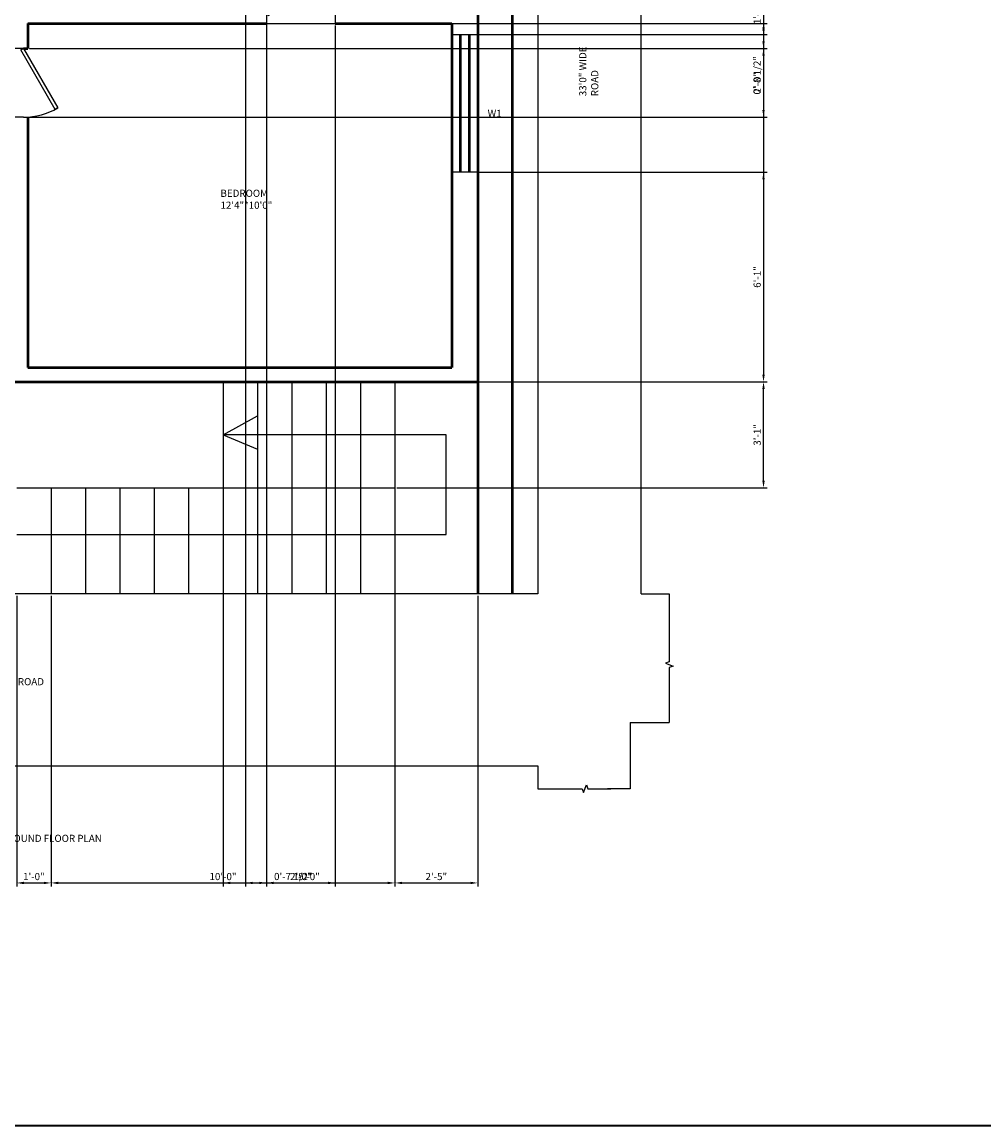
# Model space of a CAD drawing. Units: inches. Extents: x 2020 to 7901, y 1581 to 3943.
# Tile 3 of 17: x 2539 to 2875, y 1581 to 1966. Entities that reach past the tile are written whole.
import ezdxf

# ---------------------------------------------------------------- set-up
doc = ezdxf.new("R2010")
doc.units = ezdxf.units.IN
for name, color, linetype, lineweight in [('A-ANNO-DIMS', 2, 'Continuous', 18), ('A-ANNO-TEXT', 7, 'Continuous', 18), ('A-ANNO-TTLB', 7, 'Continuous', 35), ('A-AREA-IDEN', 3, 'Continuous', 18), ('A-DOOR', 4, 'Continuous', 25), ('A-FLOR-STRS', 3, 'Continuous', 25), ('A-GLAZ', 4, 'Continuous', 25), ('A-WALL', 7, 'Continuous', 50), ('C-PROP', 6, 'Continuous', 25)]:
    doc.layers.add(name, color=color, linetype=linetype, lineweight=lineweight)
doc.styles.get("Standard").update_dxf_attribs({"font": 'arial.ttf'})
doc.dimstyles.new('ISO-25', dxfattribs={"dimtxt": 2.5, "dimasz": 2.5, "dimexe": 1.25, "dimexo": 0.625, "dimtad": 1, "dimdec": 1, "dimlunit": 3, "dimtxsty": 'Standard', "dimcen": 2.5, "dimadec": 0, "dimazin": 0, "dimtfac": 1, "dimtdec": 1, "dimtmove": 0, "dimatfit": 3, "dimfxl": 1, "dimarcsym": 0})

# ---------------------------------------------------------------- blocks, each defined once
blk = doc.blocks.new('*U2')
for p, q in [((0, 0), (0, -6)), ((40, 0), (40, -6))]:
    blk.add_line(p, q)
blk.add_lwpolyline([(0, 0), (34.64, 20), (35.52, 18.48), (0.87, -1.52)], close=True)
blk.add_arc((0, 0), 40, 0, 30)
blk = doc.blocks.new('WIN-1200')
for p, q in [((0, 9), (48, 9)), ((0, 0), (0, 9)), ((48, 9), (48, 0)), ((48, 0), (0, 0))]:
    blk.add_line(p, q)
blk = doc.blocks.new('*D36')
at = {"layer": 'A-ANNO-DIMS', "color": 0, "lineweight": -2, "transparency": 16777216}
for p, q in [((2698.59, 1982.22), (2798.95, 1982.22)), ((2797.7, 1979.72), (2797.7, 1964)), ((2698.59, 1961.5), (2798.95, 1961.5))]:
    blk.add_line(p, q, dxfattribs=at)
at = {"layer": 'A-ANNO-DIMS', "color": 0, "transparency": 16777216}
for points in [[(2797.28, 1979.72), (2798.12, 1979.72), (2797.7, 1982.22)], [(2797.28, 1964), (2798.12, 1964), (2797.7, 1961.5)]]:
    blk.add_solid(points, dxfattribs=at)
at = {"layer": 'DEFPOINTS', "color": 0, "transparency": 16777216}
for p in [(2697.96, 1982.22), (2697.96, 1961.5), (2797.7, 1961.5)]:
    blk.add_point(p, dxfattribs=at)
at = {"layer": 'A-ANNO-DIMS', "color": 0, "transparency": 16777216, "insert": (2795.78, 1971.86), "char_height": 2.5, "attachment_point": 5, "rotation": 90}
blk.add_mtext('1\'-8 1/2"', dxfattribs=at)
blk = doc.blocks.new('*D37')
at = {"layer": 'A-ANNO-DIMS', "color": 0, "lineweight": -2, "transparency": 16777216}
for p, q in [((2698.59, 1913.5), (2798.95, 1913.5)), ((2797.7, 1911), (2797.7, 1842.84)), ((2698.59, 1840.34), (2798.95, 1840.34))]:
    blk.add_line(p, q, dxfattribs=at)
at = {"layer": 'A-ANNO-DIMS', "color": 0, "transparency": 16777216}
for points in [[(2797.28, 1911), (2798.12, 1911), (2797.7, 1913.5)], [(2797.28, 1842.84), (2798.12, 1842.84), (2797.7, 1840.34)]]:
    blk.add_solid(points, dxfattribs=at)
at = {"layer": 'DEFPOINTS', "color": 0, "transparency": 16777216}
for p in [(2697.96, 1913.5), (2697.96, 1840.34), (2797.7, 1840.34)]:
    blk.add_point(p, dxfattribs=at)
at = {"layer": 'A-ANNO-DIMS', "color": 0, "transparency": 16777216, "insert": (2795.8, 1876.92), "char_height": 2.5, "attachment_point": 5, "rotation": 90}
blk.add_mtext('6\'-1"', dxfattribs=at)
blk = doc.blocks.new('*D39')
at = {"layer": 'A-ANNO-DIMS', "color": 0, "lineweight": -2, "transparency": 16777216}
for p, q in [((2537.1, 1765.71), (2537.1, 1664.26)), ((2549.1, 1765.71), (2549.1, 1664.26)), ((2539.6, 1665.51), (2546.6, 1665.51))]:
    blk.add_line(p, q, dxfattribs=at)
at = {"layer": 'A-ANNO-DIMS', "color": 0, "transparency": 16777216}
for points in [[(2539.6, 1665.92), (2539.6, 1665.09), (2537.1, 1665.51)], [(2546.6, 1665.92), (2546.6, 1665.09), (2549.1, 1665.51)]]:
    blk.add_solid(points, dxfattribs=at)
at = {"layer": 'DEFPOINTS', "color": 0, "transparency": 16777216}
for p in [(2537.1, 1766.34), (2549.1, 1766.34), (2549.1, 1665.51)]:
    blk.add_point(p, dxfattribs=at)
at = {"layer": 'A-ANNO-DIMS', "color": 0, "transparency": 16777216, "insert": (2543.1, 1667.41), "char_height": 2.5, "attachment_point": 5}
blk.add_mtext('1\'-0"', dxfattribs=at)
blk = doc.blocks.new('*D40')
at = {"layer": 'A-ANNO-DIMS', "color": 0, "lineweight": -2, "transparency": 16777216}
for p, q in [((2549.1, 1765.71), (2549.1, 1664.26)), ((2669.1, 1765.71), (2669.1, 1664.26)), ((2551.6, 1665.51), (2666.6, 1665.51))]:
    blk.add_line(p, q, dxfattribs=at)
at = {"layer": 'A-ANNO-DIMS', "color": 0, "transparency": 16777216}
for points in [[(2551.6, 1665.92), (2551.6, 1665.09), (2549.1, 1665.51)], [(2666.6, 1665.92), (2666.6, 1665.09), (2669.1, 1665.51)]]:
    blk.add_solid(points, dxfattribs=at)
at = {"layer": 'DEFPOINTS', "color": 0, "transparency": 16777216}
for p in [(2549.1, 1766.34), (2669.1, 1766.34), (2669.1, 1665.51)]:
    blk.add_point(p, dxfattribs=at)
at = {"layer": 'A-ANNO-DIMS', "color": 0, "transparency": 16777216, "insert": (2609.1, 1667.41), "char_height": 2.5, "attachment_point": 5}
blk.add_mtext('10\'-0"', dxfattribs=at)
blk = doc.blocks.new('*D96')
at = {"layer": 'A-ANNO-DIMS', "color": 0, "lineweight": -2, "transparency": 16777216}
for p, q in [((2698.59, 2214.34), (2798.95, 2214.34)), ((2797.7, 2211.84), (2797.7, 1842.84)), ((2698.59, 1840.34), (2798.95, 1840.34))]:
    blk.add_line(p, q, dxfattribs=at)
at = {"layer": 'A-ANNO-DIMS', "color": 0, "transparency": 16777216}
for points in [[(2797.28, 2211.84), (2798.12, 2211.84), (2797.7, 2214.34)], [(2797.28, 1842.84), (2798.12, 1842.84), (2797.7, 1840.34)]]:
    blk.add_solid(points, dxfattribs=at)
at = {"layer": 'DEFPOINTS', "color": 0, "transparency": 16777216}
for p in [(2697.96, 2214.34), (2697.96, 1840.34), (2797.7, 1840.34)]:
    blk.add_point(p, dxfattribs=at)
at = {"layer": 'A-ANNO-DIMS', "color": 0, "transparency": 16777216, "insert": (2795.8, 2027.34), "char_height": 2.5, "attachment_point": 5, "rotation": 90}
blk.add_mtext('31\'-2"', dxfattribs=at)
blk = doc.blocks.new('*D112')
at = {"layer": 'A-ANNO-DIMS', "color": 0, "lineweight": -2, "transparency": 16777216}
for p, q in [((2541.59, 1965.34), (2798.95, 1965.34)), ((2797.7, 1962.84), (2797.7, 1959.17)), ((2541.59, 1956.67), (2798.95, 1956.67)), ((2797.7, 1956.67), (2797.7, 1940.45))]:
    blk.add_line(p, q, dxfattribs=at)
at = {"layer": 'A-ANNO-DIMS', "color": 0, "transparency": 16777216}
for points in [[(2797.28, 1962.84), (2798.12, 1962.84), (2797.7, 1965.34)], [(2797.28, 1959.17), (2798.12, 1959.17), (2797.7, 1956.67)]]:
    blk.add_solid(points, dxfattribs=at)
at = {"layer": 'DEFPOINTS', "color": 0, "transparency": 16777216}
for p in [(2540.96, 1965.34), (2540.96, 1956.67), (2797.7, 1956.67)]:
    blk.add_point(p, dxfattribs=at)
at = {"layer": 'A-ANNO-DIMS', "color": 0, "transparency": 16777216, "insert": (2795.78, 1947.31), "char_height": 2.5, "attachment_point": 5, "rotation": 90}
blk.add_mtext('0\'-8 1/2"', dxfattribs=at)
blk = doc.blocks.new('*D113')
at = {"layer": 'A-ANNO-DIMS', "color": 0, "lineweight": -2, "transparency": 16777216}
for p, q in [((2541.59, 1956.67), (2798.95, 1956.67)), ((2797.7, 1954.17), (2797.7, 1935.21)), ((2541.59, 1932.71), (2798.95, 1932.71))]:
    blk.add_line(p, q, dxfattribs=at)
at = {"layer": 'A-ANNO-DIMS', "color": 0, "transparency": 16777216}
for points in [[(2797.28, 1954.17), (2798.12, 1954.17), (2797.7, 1956.67)], [(2797.28, 1935.21), (2798.12, 1935.21), (2797.7, 1932.71)]]:
    blk.add_solid(points, dxfattribs=at)
at = {"layer": 'DEFPOINTS', "color": 0, "transparency": 16777216}
for p in [(2540.96, 1956.67), (2540.96, 1932.71), (2797.7, 1932.71)]:
    blk.add_point(p, dxfattribs=at)
at = {"layer": 'A-ANNO-DIMS', "color": 0, "transparency": 16777216, "insert": (2795.8, 1944.69), "char_height": 2.5, "attachment_point": 5, "rotation": 90}
blk.add_mtext('2\'-0"', dxfattribs=at)
blk = doc.blocks.new('*D116')
at = {"layer": 'A-ANNO-DIMS', "color": 0, "lineweight": -2, "transparency": 16777216}
for p, q in [((2616.96, 1969.71), (2616.96, 1664.26)), ((2624.26, 1969.71), (2624.26, 1664.26)), ((2619.46, 1665.51), (2621.76, 1665.51)), ((2624.26, 1665.51), (2640.48, 1665.51))]:
    blk.add_line(p, q, dxfattribs=at)
at = {"layer": 'A-ANNO-DIMS', "color": 0, "transparency": 16777216}
for points in [[(2619.46, 1665.92), (2619.46, 1665.09), (2616.96, 1665.51)], [(2621.76, 1665.92), (2621.76, 1665.09), (2624.26, 1665.51)]]:
    blk.add_solid(points, dxfattribs=at)
at = {"layer": 'DEFPOINTS', "color": 0, "transparency": 16777216}
for p in [(2616.96, 1970.34), (2624.26, 1970.34), (2624.26, 1665.51)]:
    blk.add_point(p, dxfattribs=at)
at = {"layer": 'A-ANNO-DIMS', "color": 0, "transparency": 16777216, "insert": (2633.62, 1667.43), "char_height": 2.5, "attachment_point": 5}
blk.add_mtext('0\'-7 1/2"', dxfattribs=at)
blk = doc.blocks.new('*D117')
at = {"layer": 'A-ANNO-DIMS', "color": 0, "lineweight": -2, "transparency": 16777216}
for p, q in [((2624.26, 1964.71), (2624.26, 1664.26)), ((2648.26, 1964.71), (2648.26, 1664.26)), ((2626.76, 1665.51), (2645.76, 1665.51))]:
    blk.add_line(p, q, dxfattribs=at)
at = {"layer": 'A-ANNO-DIMS', "color": 0, "transparency": 16777216}
for points in [[(2626.76, 1665.92), (2626.76, 1665.09), (2624.26, 1665.51)], [(2645.76, 1665.92), (2645.76, 1665.09), (2648.26, 1665.51)]]:
    blk.add_solid(points, dxfattribs=at)
at = {"layer": 'DEFPOINTS', "color": 0, "transparency": 16777216}
for p in [(2624.26, 1965.34), (2648.26, 1965.34), (2648.26, 1665.51)]:
    blk.add_point(p, dxfattribs=at)
at = {"layer": 'A-ANNO-DIMS', "color": 0, "transparency": 16777216, "insert": (2636.26, 1667.41), "char_height": 2.5, "attachment_point": 5}
blk.add_mtext('2\'-0"', dxfattribs=at)
blk = doc.blocks.new('*D119')
at = {"layer": 'A-ANNO-DIMS', "color": 0, "lineweight": -2, "transparency": 16777216}
for p, q in [((2609.1, 1839.71), (2609.1, 1664.26)), ((2669.1, 1839.71), (2669.1, 1664.26)), ((2611.6, 1665.51), (2666.6, 1665.51))]:
    blk.add_line(p, q, dxfattribs=at)
at = {"layer": 'A-ANNO-DIMS', "color": 0, "transparency": 16777216}
for points in [[(2611.6, 1665.92), (2611.6, 1665.09), (2609.1, 1665.51)], [(2666.6, 1665.92), (2666.6, 1665.09), (2669.1, 1665.51)]]:
    blk.add_solid(points, dxfattribs=at)
at = {"layer": 'DEFPOINTS', "color": 0, "transparency": 16777216}
for p in [(2609.1, 1840.34), (2669.1, 1840.34), (2669.1, 1665.51)]:
    blk.add_point(p, dxfattribs=at)
at = {"layer": 'A-ANNO-DIMS', "color": 0, "transparency": 16777216, "insert": (2639.1, 1667.41), "char_height": 2.5, "attachment_point": 5}
blk.add_mtext('5\'-0"', dxfattribs=at)
blk = doc.blocks.new('*D120')
at = {"layer": 'A-ANNO-DIMS', "color": 0, "lineweight": -2, "transparency": 16777216}
for p, q in [((2669.73, 1840.34), (2798.95, 1840.34)), ((2797.7, 1805.84), (2797.7, 1837.84)), ((2669.73, 1803.34), (2798.95, 1803.34))]:
    blk.add_line(p, q, dxfattribs=at)
at = {"layer": 'A-ANNO-DIMS', "color": 0, "transparency": 16777216}
for points in [[(2797.28, 1837.84), (2798.12, 1837.84), (2797.7, 1840.34)], [(2797.28, 1805.84), (2798.12, 1805.84), (2797.7, 1803.34)]]:
    blk.add_solid(points, dxfattribs=at)
at = {"layer": 'DEFPOINTS', "color": 0, "transparency": 16777216}
for p in [(2669.1, 1840.34), (2797.7, 1840.34), (2669.1, 1803.34)]:
    blk.add_point(p, dxfattribs=at)
at = {"layer": 'A-ANNO-DIMS', "color": 0, "transparency": 16777216, "insert": (2795.8, 1821.84), "char_height": 2.5, "attachment_point": 5, "rotation": 90}
blk.add_mtext('3\'-1"', dxfattribs=at)
blk = doc.blocks.new('*D121')
at = {"layer": 'A-ANNO-DIMS', "color": 0, "lineweight": -2, "transparency": 16777216}
for p, q in [((2669.1, 1765.71), (2669.1, 1664.26)), ((2697.96, 1765.71), (2697.96, 1664.26)), ((2671.6, 1665.51), (2695.46, 1665.51))]:
    blk.add_line(p, q, dxfattribs=at)
at = {"layer": 'A-ANNO-DIMS', "color": 0, "transparency": 16777216}
for points in [[(2671.6, 1665.92), (2671.6, 1665.09), (2669.1, 1665.51)], [(2695.46, 1665.92), (2695.46, 1665.09), (2697.96, 1665.51)]]:
    blk.add_solid(points, dxfattribs=at)
at = {"layer": 'DEFPOINTS', "color": 0, "transparency": 16777216}
for p in [(2669.1, 1766.34), (2697.96, 1766.34), (2697.96, 1665.51)]:
    blk.add_point(p, dxfattribs=at)
at = {"layer": 'A-ANNO-DIMS', "color": 0, "transparency": 16777216, "insert": (2683.53, 1667.41), "char_height": 2.5, "attachment_point": 5}
blk.add_mtext('2\'-5"', dxfattribs=at)

msp = doc.modelspace()

# ---------------------------------------------------------------- linework, layer by layer
at = {"layer": 'A-ANNO-TTLB'}
msp.add_lwpolyline([(2019.8, 3067.25), (4199.03, 3067.25), (4199.03, 1580.73), (2019.8, 1580.73)], close=True, dxfattribs=at)
at = {"layer": 'A-FLOR-STRS'}
for p, q in [((2609.1, 1840.34), (2609.1, 1766.34)), ((2621.1, 1840.34), (2621.1, 1766.34)), ((2633.1, 1840.34), (2633.1, 1766.34)), ((2645.1, 1840.34), (2645.1, 1766.34)), ((2657.1, 1840.34), (2657.1, 1766.34)), ((2669.1, 1840.34), (2669.1, 1766.34)), ((2609.1, 1821.84), (2621.1, 1828.53)), ((2686.94, 1821.84), (2609.1, 1821.84)), ((2609.1, 1821.84), (2621.1, 1816.89)), ((2686.94, 1787.09), (2686.94, 1821.84)), ((2537.1, 1803.34), (2669.1, 1803.34)), ((2549.1, 1803.34), (2549.1, 1766.34)), ((2561.1, 1803.34), (2561.1, 1766.34)), ((2573.1, 1803.34), (2573.1, 1766.34)), ((2585.1, 1803.34), (2585.1, 1766.34)), ((2597.1, 1803.34), (2597.1, 1766.34)), ((2537.1, 1787.09), (2686.94, 1787.09))]:
    msp.add_line(p, q, dxfattribs=at)
at = {"layer": 'A-WALL'}
for p, q in [((2709.96, 2237.34), (2709.96, 1766.34)), ((2697.96, 2214.34), (2697.96, 1766.34)), ((2540.96, 1965.34), (2624.26, 1965.34)), ((2540.96, 1965.34), (2540.96, 1956.67)), ((2648.26, 1965.34), (2688.96, 1965.34)), ((2688.96, 1965.34), (2688.96, 1845.34)), ((2691.96, 1913.5), (2691.96, 1961.5)), ((2694.96, 1961.5), (2694.96, 1913.5)), ((2539.5, 1956.67), (2540.96, 1956.67)), ((2540.96, 1932.71), (2540.96, 1845.34)), ((2540.96, 1845.34), (2688.96, 1845.34)), ((2535.96, 1840.34), (2697.96, 1840.34))]:
    msp.add_line(p, q, dxfattribs=at)
at = {"layer": 'C-PROP'}
for p, q in [((2754.96, 1766.34), (2754.96, 2276.61)), ((2718.96, 2246.34), (2718.96, 1766.34)), ((2718.96, 1766.34), (2358.96, 1766.34)), ((2754.96, 1766.34), (2764.83, 1766.34)), ((2754.96, 1766.34), (2764.83, 1766.34)), ((2764.83, 1766.34), (2764.83, 1758.09)), ((2764.83, 1758.09), (2764.83, 1742.64)), ((2764.83, 1740.64), (2764.83, 1721.47)), ((2751.2, 1721.47), (2764.83, 1721.47)), ((2751.2, 1721.47), (2751.2, 1698.38)), ((2349.95, 1706.34), (2718.96, 1706.34)), ((2718.96, 1706.34), (2718.96, 1698.38)), ((2718.96, 1698.38), (2727.64, 1698.38)), ((2751.2, 1698.38), (2743.2, 1698.38))]:
    msp.add_line(p, q, dxfattribs=at)
for points in [[(2764.83, 1751.4), (2764.83, 1742.64), (2763.45, 1742.14), (2766.2, 1741.14), (2764.83, 1740.64), (2764.83, 1731.88)], [(2726.39, 1698.38), (2734.42, 1698.38), (2734.92, 1697.01), (2735.92, 1699.76), (2736.42, 1698.38), (2744.45, 1698.38)]]:
    msp.add_lwpolyline(points, dxfattribs=at)

# ---------------------------------------------------------------- block references
at = {"layer": 'A-DOOR', "xscale": 0.6, "yscale": 0.6, "zscale": 0.6}
msp.add_blockref('*U2', (2624.26, 1968.92), dxfattribs=at)
at = {"layer": 'A-DOOR', "xscale": 0.6, "yscale": 0.6, "zscale": 0.6, "rotation": 270}
msp.add_blockref('*U2', (2539.5, 1956.67), dxfattribs=at)
at = {"layer": 'A-GLAZ', "rotation": 89.99999999999991}
msp.add_blockref('WIN-1200', (2697.97, 1913.5), dxfattribs=at)

# ---------------------------------------------------------------- texts
at = {"layer": 'A-ANNO-TEXT', "insert": (2733.38, 1939.99), "char_height": 2.5, "attachment_point": 1, "rotation": 90}
msp.add_mtext_dynamic_manual_height_columns('33\'0" WIDE  ROAD', width=23.8844, gutter_width=12.5, heights=[0], dxfattribs=at)
at = {"layer": 'A-ANNO-TEXT', "char_height": 2.5, "attachment_point": 1}
for s, width, insert in [('W1', 7.8806, (2701.44, 1935.25)), ('25\'0"  WIDE  ROAD', 215.7208, (2517.86, 1736.97)), ('GROUND FLOOR PLAN', 228.0251, (2531.45, 1682.31))]:
    msp.add_mtext_dynamic_manual_height_columns(s, width=width, gutter_width=12.5, heights=[0], dxfattribs=dict(at, insert=insert))
at = {"layer": 'A-AREA-IDEN', "insert": (2608.22, 1907.38), "char_height": 2.5, "attachment_point": 1}
msp.add_mtext_dynamic_manual_height_columns('BEDROOM\\P12\'4"*10\'0"', width=71.6344, gutter_width=12.5, heights=[0], dxfattribs=at)

# ---------------------------------------------------------------- dimensions: what is measured, and where the dimension line sits
at = {"layer": 'A-ANNO-DIMS'}
for base, p1, p2, picture, middle in [((2797.7, 1840.34), (2697.96, 2214.34), (2697.96, 1840.34), '*D96', (2795.8, 2027.34)), ((2797.7, 1961.5), (2697.96, 1982.22), (2697.96, 1961.5), '*D36', (2795.78, 1971.86)), ((2797.7, 1956.67), (2540.96, 1965.34), (2540.96, 1956.67), '*D112', (2795.78, 1947.31)), ((2797.7, 1932.71), (2540.96, 1956.67), (2540.96, 1932.71), '*D113', (2795.8, 1944.69)), ((2797.7, 1840.34), (2697.96, 1913.5), (2697.96, 1840.34), '*D37', (2795.8, 1876.92)), ((2797.7, 1840.34), (2669.1, 1803.34), (2669.1, 1840.34), '*D120', (2795.8, 1821.84))]:
    dim = msp.add_linear_dim(base=base, p1=p1, p2=p2, angle=90, dimstyle='ISO-25', override={"dimdec": 1, "dimlfac": 1, "dimrnd": 0, "dimzin": 1, "dimdsep": 46, "dimlunit": 4, "dimfrac": 2}, dxfattribs=at)
    dim.commit()
    dim.dimension.update_dxf_attribs({"geometry": picture, "text_midpoint": middle})
for base, p1, p2, picture, middle in [((2624.26, 1665.51), (2616.96, 1970.34), (2624.26, 1970.34), '*D116', (2633.62, 1667.43)), ((2648.26, 1665.51), (2624.26, 1965.34), (2648.26, 1965.34), '*D117', (2636.26, 1667.41)), ((2669.1, 1665.51), (2609.1, 1840.34), (2669.1, 1840.34), '*D119', (2639.1, 1667.41)), ((2549.1, 1665.51), (2537.1, 1766.34), (2549.1, 1766.34), '*D39', (2543.1, 1667.41)), ((2669.1, 1665.51), (2549.1, 1766.34), (2669.1, 1766.34), '*D40', (2609.1, 1667.41)), ((2697.96, 1665.51), (2669.1, 1766.34), (2697.96, 1766.34), '*D121', (2683.53, 1667.41))]:
    dim = msp.add_linear_dim(base=base, p1=p1, p2=p2, dimstyle='ISO-25', override={"dimdec": 1, "dimlfac": 1, "dimrnd": 0, "dimzin": 1, "dimdsep": 46, "dimlunit": 4, "dimfrac": 2}, dxfattribs=at)
    dim.commit()
    dim.dimension.update_dxf_attribs({"geometry": picture, "text_midpoint": middle})

doc.saveas('drawing.dxf')
